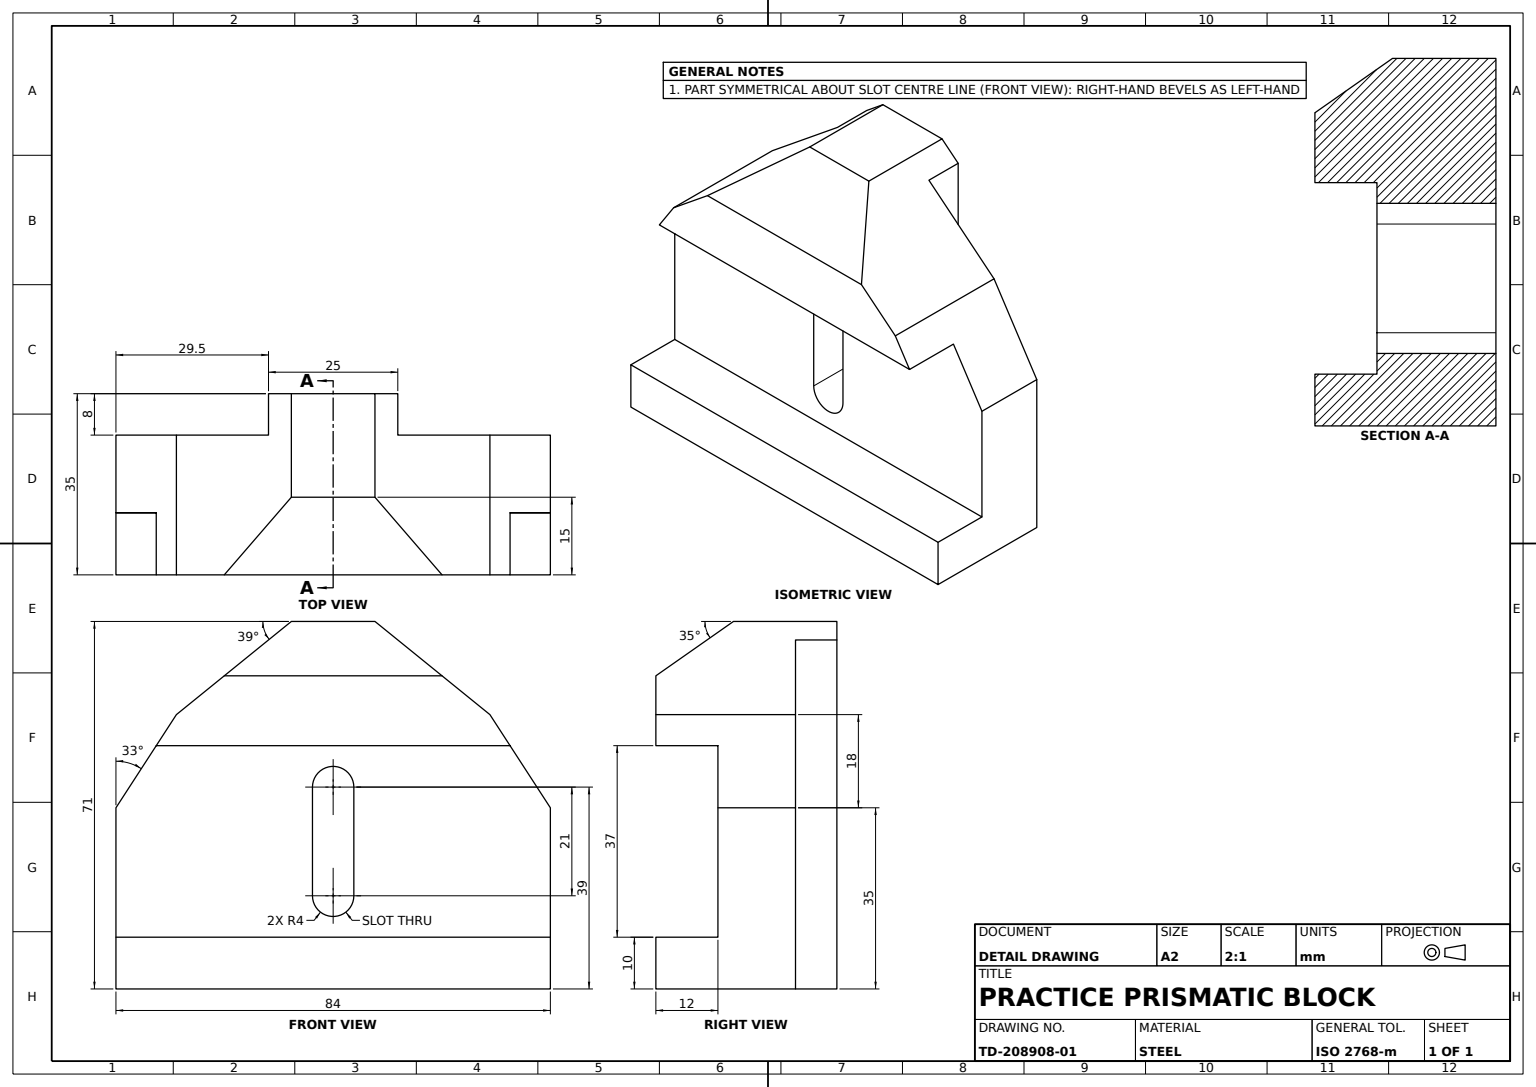
from build123d import *

# Parameters (mm, degrees)
SUPPORT_BLOCK_84MM_DEPTH = 84
TOP_BEVEL_CUT_DEPTH      = 84
SLOT_8MM_SKETCH_W        = 29.5
SLOT_8MM_SKETCH_H        = 8
SLOT_8MM_CUT_DEPTH       = 104
SLOT_8X21_CUT_DEPTH      = 104


with BuildPart() as part:
    # Block Profile Sketch → Support Block 84mm (new body)
    with BuildSketch(Plane(origin=(0, 0, 0), x_dir=(0, 0, -1), z_dir=(1, 0, 0))):
        Polygon((-23, 47), (-23, 10), (-35, 10), (-35, 0), (0, 0), (0, 71), (-20, 71), (-35, 60.496886927), (-35, 47), align=None)
    extrude(amount=-SUPPORT_BLOCK_84MM_DEPTH)

    # Top Bevel Sketch → Top Bevel Cut (cut)
    with BuildSketch(Plane.XY.offset(35)):
        Polygon((0, 35), (-11.689336678, 53), (-33.917485495, 71), (24.610458678, 71), (24.610458678, 35), align=None)
        Polygon((-50.082514505, 71), (-95.876326583, 71), (-95.876326583, 33.772958176), (-84, 35), (-72.310663322, 53), align=None)
    extrude(amount=-TOP_BEVEL_CUT_DEPTH, mode=Mode.SUBTRACT)

    # Slot 8mm Sketch → Slot 8mm Cut (cut)
    with BuildSketch(Plane(origin=(0, 71, 0), x_dir=(1, 0, 0), z_dir=(0, 1, 0))):
        with Locations((-69.25, -4)):
            Rectangle(SLOT_8MM_SKETCH_W, SLOT_8MM_SKETCH_H)
        with Locations((-14.75, -4)):
            Rectangle(SLOT_8MM_SKETCH_W, SLOT_8MM_SKETCH_H)
    extrude(amount=-SLOT_8MM_CUT_DEPTH, mode=Mode.SUBTRACT)

    # Slot 8x21 Sketch → Slot 8x21 Cut (cut)
    with BuildSketch(Plane.XY.offset(23)):
        with BuildLine():
            Line((-46, 18), (-46, 39))
            ThreePointArc((-46, 39), (-42, 43), (-38, 39))
            Line((-38, 39), (-38, 18))
            ThreePointArc((-38, 18), (-42, 14), (-46, 18))
        make_face()
    extrude(amount=-SLOT_8X21_CUT_DEPTH, mode=Mode.SUBTRACT)


solid = part.part
